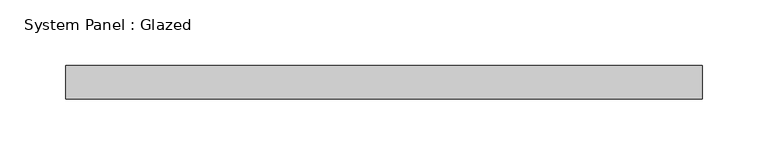
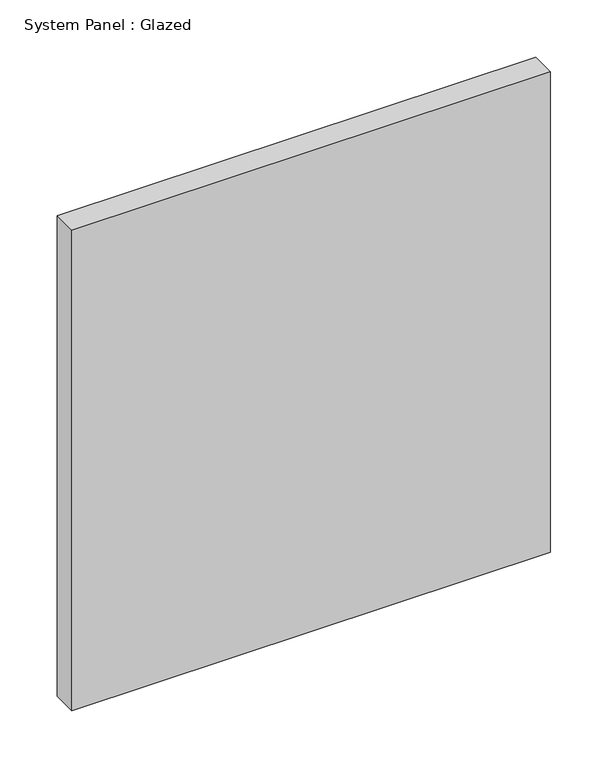
"""IFC4 building model written with IfcOpenShell, lengths in millimetres: plate geometry, System Panel : Glazed."""

from ifc_helpers import new_model, si_unit, origin, origin_with_axes, place, context, project, spatial, polyline, outline, extrude, source, transform, mapped, element, save


def system_panel_glazed_84c2177b(model_context):
    return source(origin(), model_context, "Body", "SweptSolid", [
        extrude(outline(polyline([(241.3, 19.05), (-241.3, 19.05), (-241.3, 44.45), (241.3, 44.45), (241.3, 19.05)])), origin_with_axes(), (0.0, 0.0, 1.0), 512.3872143),
    ])


if __name__ == "__main__":
    model = new_model("IFC4")
    model_context = context("Model", 3, world=origin())
    ifc_project = project(units=[si_unit("LENGTHUNIT", "METRE", prefix="MILLI")], contexts=[model_context])
    site = spatial("IfcSite", under=ifc_project)
    building = spatial("IfcBuilding", under=site)
    placement = place(None, origin())
    system_panel_glazed_shape = system_panel_glazed_84c2177b(model_context)
    element("IfcPlate", 1, ObjectType="System Panel : Glazed", at=placement, inside=building, context=model_context, shape_type="MappedRepresentation", body=[
        mapped(system_panel_glazed_shape, transform((0.0, 0.0, 0.0), x_axis=(1.0, 0.0, 0.0), y_axis=(0.0, 1.0, 0.0), z_axis=(0.0, 0.0, 1.0))),
    ])
    save(model, "model.ifc")

# Revit data of these elements
# Type "System Panel : Glazed"
#   Construction Type Id = "GSP4R"
#   Analytic Construction = "1/8 in Pilkington single glazing"
#   Visual Light Transmittance = 0.9
#   Solar Heat Gain Coefficient = 0.86
#   Heat Transfer Coefficient (U) = 1.18115 BTU/(h·ft²·°F)
#   Define Thermal Properties by = 1
# Element 1 (IfcPlate, "System Panel : Glazed")
#   Materials on its faces: "Glass"
# Materials
#   "Glass": class "Glass", colour RGB 0 128 192, transparency 0.75, Description = "Soda Lime Glass", Cost = 0
